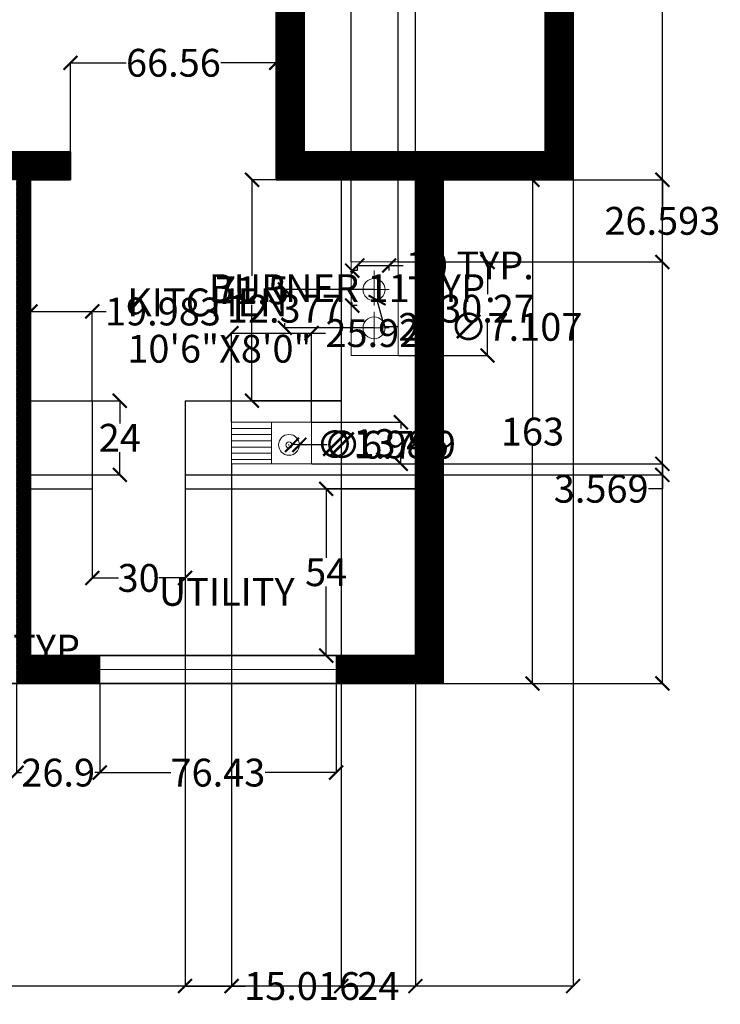
# Model space of a CAD drawing. Units: inches. Extents: x -124 to 468, y -83 to 563.
# Tile 2 of 3: x 241 to 468, y -83 to 235. Entities that reach past the tile are written whole.
import ezdxf

# ---------------------------------------------------------------- set-up
doc = ezdxf.new("R2010")
doc.units = ezdxf.units.IN
doc.header["$MEASUREMENT"] = 0
for name, color, linetype, lineweight in [('A-ANNO-DIMS', 2, 'Continuous', 18), ('A-AREA-IDEN', 7, 'Continuous', 18), ('A-EQPM', 8, 'Continuous', 18), ('A-FLOR-FIXT', 8, 'Continuous', 18)]:
    doc.layers.add(name, color=color, linetype=linetype, lineweight=lineweight)
for name, color, linetype, lineweight, true_color in [('A-FLOR-CASE', 35, 'Continuous', 25, 0x836e59), ('A-GLAZ', 145, 'Continuous', 18, 0x2a88b7), ('A-WALL', 149, 'Continuous', 35, 0x414448), ('A-WALL-PATT', 251, 'Continuous', 13, 0x585a5e)]:
    doc.layers.add(name, color=color, linetype=linetype, lineweight=lineweight, true_color=true_color)
doc.styles.get("Standard").update_dxf_attribs({"font": 'arial.ttf'})
doc.dimstyles.get("Standard").update_dxf_attribs({"dimtxt": 9, "dimasz": 4.5, "dimexe": 0.18, "dimexo": 0.0625, "dimgap": 0.09, "dimtad": 0, "dimtih": 1, "dimtoh": 1, "dimdec": 1, "dimzin": 0, "dimdsep": 46, "dimlunit": 4, "dimtxsty": 'Standard', "dimblk": 'ARCHTICK', "dimcen": 0.09, "dimadec": 0, "dimazin": 0, "dimtfac": 1, "dimtdec": 1, "dimtofl": 0, "dimtmove": 0, "dimatfit": 3, "dimfxl": 1, "dimtolj": 1, "dimtzin": 0, "dimarcsym": 0})

# ---------------------------------------------------------------- blocks, each defined once
blk = doc.blocks.new('COOKTOP-BURNER')
for p, q in [((5.38, 5.19), (5.38, 11.31)), ((5.38, 11.31), (5.38, 5.19)), ((5.38, 5.19), (0, 5.19)), ((5.38, 5.19), (10.26, 5.19)), ((10.26, 5.19), (5.38, 5.19)), ((5.38, 5.19), (5.38, 0)), ((5.38, 0), (5.38, 5.19))]:
    blk.add_line(p, q)
blk.add_circle((5.38, 5.19), 3.55)
blk = doc.blocks.new('_ArchTick')
at = {"color": 0, "linetype": 'ByBlock', "const_width": 0.15}
blk.add_lwpolyline([(-0.5, -0.5), (0.5, 0.5)], dxfattribs=at)
blk = doc.blocks.new('*D6')
at = {"layer": 'A-ANNO-DIMS', "color": 0, "lineweight": -2, "transparency": 16777216}
for p, q in [((39.84, 46.01), (39.84, 31.49)), ((135.84, 46.01), (135.84, 31.49)), ((39.84, 31.67), (135.84, 31.67)), ((135.84, 31.67), (140.34, 31.67))]:
    blk.add_line(p, q, dxfattribs=at)
at = {"layer": 'Defpoints', "color": 0, "transparency": 16777216}
for p in [(39.84, 46.07), (135.84, 46.07), (135.84, 31.67)]:
    blk.add_point(p, dxfattribs=at)
at = {"layer": 'A-ANNO-DIMS', "color": 0, "lineweight": -2, "transparency": 16777216, "xscale": 4.5, "yscale": 4.5, "zscale": 4.5, "rotation": 180}
blk.add_blockref('_ArchTick', (39.84, 31.67), dxfattribs=at)
at = {"layer": 'A-ANNO-DIMS', "color": 0, "lineweight": -2, "transparency": 16777216, "xscale": 4.5, "yscale": 4.5, "zscale": 4.5}
blk.add_blockref('_ArchTick', (135.84, 31.67), dxfattribs=at)
at = {"layer": 'A-ANNO-DIMS', "color": 0, "transparency": 16777216, "insert": (204.38, 31.67), "char_height": 9, "attachment_point": 5}
blk.add_mtext('\\A1;DOUBLE BED 96 TYP.', dxfattribs=at)
blk = doc.blocks.new('*D12')
at = {"layer": 'A-ANNO-DIMS', "color": 0, "lineweight": -2, "transparency": 16777216}
for p, q in [((350.16, 153.98), (348.34, 153.98)), ((348.52, 153.98), (348.52, 153.01)), ((348.52, 142.67), (348.52, 143.64)), ((350.16, 142.67), (348.34, 142.67))]:
    blk.add_line(p, q, dxfattribs=at)
at = {"layer": 'Defpoints', "color": 0, "transparency": 16777216}
for p in [(348.52, 153.98), (350.22, 153.98), (350.22, 142.67)]:
    blk.add_point(p, dxfattribs=at)
at = {"layer": 'A-ANNO-DIMS', "color": 0, "lineweight": -2, "transparency": 16777216, "xscale": 4.5, "yscale": 4.5, "zscale": 4.5}
for p, rotation in [((348.52, 153.98), 90), ((348.52, 142.67), 270)]:
    blk.add_blockref('_ArchTick', p, dxfattribs=dict(at, rotation=rotation))
at = {"layer": 'A-ANNO-DIMS', "color": 0, "transparency": 16777216, "insert": (348.52, 148.32), "char_height": 9, "attachment_point": 5}
blk.add_mtext('\\A1;BURNER 11 TYP.', dxfattribs=at)
blk = doc.blocks.new('*D13')
at = {"layer": 'A-ANNO-DIMS', "color": 0, "lineweight": -2, "transparency": 16777216}
for p, q in [((350.22, 154.04), (350.22, 155.86)), ((350.22, 155.68), (360.48, 155.68)), ((360.48, 154.04), (360.48, 155.86)), ((360.48, 155.68), (364.98, 155.68))]:
    blk.add_line(p, q, dxfattribs=at)
at = {"layer": 'Defpoints', "color": 0, "transparency": 16777216}
for p in [(350.22, 153.98), (360.48, 155.68), (360.48, 153.98)]:
    blk.add_point(p, dxfattribs=at)
at = {"layer": 'A-ANNO-DIMS', "color": 0, "lineweight": -2, "transparency": 16777216, "xscale": 4.5, "yscale": 4.5, "zscale": 4.5, "rotation": 180}
blk.add_blockref('_ArchTick', (350.22, 155.68), dxfattribs=at)
at = {"layer": 'A-ANNO-DIMS', "color": 0, "lineweight": -2, "transparency": 16777216, "xscale": 4.5, "yscale": 4.5, "zscale": 4.5}
blk.add_blockref('_ArchTick', (360.48, 155.68), dxfattribs=at)
at = {"layer": 'A-ANNO-DIMS', "color": 0, "transparency": 16777216, "insert": (386.55, 155.68), "char_height": 9, "attachment_point": 5}
blk.add_mtext('\\A1;10 TYP.', dxfattribs=at)
blk = doc.blocks.new('*D14')
at = {"layer": 'A-ANNO-DIMS', "color": 0, "lineweight": -2, "transparency": 16777216}
for p, q in [((419.98, 183.33), (419.98, -77.73)), ((-79.52, -48.75), (-79.52, -77.73)), ((-79.52, -77.55), (154.74, -77.55)), ((419.98, -77.55), (185.72, -77.55))]:
    blk.add_line(p, q, dxfattribs=at)
at = {"layer": 'Defpoints', "color": 0, "transparency": 16777216}
for p in [(419.98, 183.39), (-79.52, -48.69), (419.98, -77.55)]:
    blk.add_point(p, dxfattribs=at)
at = {"layer": 'A-ANNO-DIMS', "color": 0, "lineweight": -2, "transparency": 16777216, "xscale": 4.5, "yscale": 4.5, "zscale": 4.5, "rotation": 180}
blk.add_blockref('_ArchTick', (-79.52, -77.55), dxfattribs=at)
at = {"layer": 'A-ANNO-DIMS', "color": 0, "lineweight": -2, "transparency": 16777216, "xscale": 4.5, "yscale": 4.5, "zscale": 4.5}
blk.add_blockref('_ArchTick', (419.98, -77.55), dxfattribs=at)
at = {"layer": 'A-ANNO-DIMS', "color": 0, "transparency": 16777216, "insert": (170.23, -77.55), "char_height": 9, "attachment_point": 5}
blk.add_mtext('\\A1;499.5', dxfattribs=at)
blk = doc.blocks.new('*D17')
at = {"layer": 'A-ANNO-DIMS', "color": 0, "lineweight": -2, "transparency": 16777216}
for p, q in [((378.04, 486.39), (449.02, 486.39)), ((448.84, 486.39), (448.84, 258.08)), ((448.84, 20.39), (448.84, 248.71)), ((378.04, 20.39), (449.02, 20.39))]:
    blk.add_line(p, q, dxfattribs=at)
at = {"layer": 'Defpoints', "color": 0, "transparency": 16777216}
for p in [(377.98, 486.39), (448.84, 486.39), (377.98, 20.39)]:
    blk.add_point(p, dxfattribs=at)
at = {"layer": 'A-ANNO-DIMS', "color": 0, "lineweight": -2, "transparency": 16777216, "xscale": 4.5, "yscale": 4.5, "zscale": 4.5}
for p, rotation in [((448.84, 486.39), 90), ((448.84, 20.39), 270)]:
    blk.add_blockref('_ArchTick', p, dxfattribs=dict(at, rotation=rotation))
at = {"layer": 'A-ANNO-DIMS', "color": 0, "transparency": 16777216, "insert": (448.84, 253.39), "char_height": 9, "attachment_point": 5}
blk.add_mtext('\\A1;466', dxfattribs=at)
blk = doc.blocks.new('*D21')
at = {"layer": 'A-ANNO-DIMS', "color": 0, "lineweight": -2, "transparency": 16777216}
for p, q in [((378.04, 183.39), (407.02, 183.39)), ((406.84, 183.39), (406.84, 106.58)), ((406.84, 20.39), (406.84, 97.2)), ((378.04, 20.39), (407.02, 20.39))]:
    blk.add_line(p, q, dxfattribs=at)
at = {"layer": 'Defpoints', "color": 0, "transparency": 16777216}
for p in [(377.98, 183.39), (377.98, 20.39), (406.84, 20.39)]:
    blk.add_point(p, dxfattribs=at)
at = {"layer": 'A-ANNO-DIMS', "color": 0, "lineweight": -2, "transparency": 16777216, "xscale": 4.5, "yscale": 4.5, "zscale": 4.5}
for p, rotation in [((406.84, 183.39), 90), ((406.84, 20.39), 270)]:
    blk.add_blockref('_ArchTick', p, dxfattribs=dict(at, rotation=rotation))
at = {"layer": 'A-ANNO-DIMS', "color": 0, "transparency": 16777216, "insert": (406.84, 101.89), "char_height": 9, "attachment_point": 5}
blk.add_mtext('\\A1;163', dxfattribs=at)
blk = doc.blocks.new('*D31')
at = {"layer": 'A-ANNO-DIMS', "color": 0, "lineweight": -2, "transparency": 16777216}
for p, q in [((239.98, 20.33), (239.98, -8.65)), ((266.88, 20.33), (266.88, -8.65)), ((239.98, -8.47), (241.56, -8.47)), ((266.88, -8.47), (265.29, -8.47))]:
    blk.add_line(p, q, dxfattribs=at)
at = {"layer": 'Defpoints', "color": 0, "transparency": 16777216}
for p in [(239.98, 20.39), (266.88, 20.39), (239.98, -8.47)]:
    blk.add_point(p, dxfattribs=at)
at = {"layer": 'A-ANNO-DIMS', "color": 0, "lineweight": -2, "transparency": 16777216, "xscale": 4.5, "yscale": 4.5, "zscale": 4.5, "rotation": 180.0000000000002}
blk.add_blockref('_ArchTick', (239.98, -8.47), dxfattribs=at)
at = {"layer": 'A-ANNO-DIMS', "color": 0, "lineweight": -2, "transparency": 16777216, "xscale": 4.5, "yscale": 4.5, "zscale": 4.5}
blk.add_blockref('_ArchTick', (266.88, -8.47), dxfattribs=at)
at = {"layer": 'A-ANNO-DIMS', "color": 0, "transparency": 16777216, "insert": (253.43, -8.47), "char_height": 9, "attachment_point": 5}
blk.add_mtext('\\A1;26.9', dxfattribs=at)
blk = doc.blocks.new('*D32')
at = {"layer": 'A-ANNO-DIMS', "color": 0, "lineweight": -2, "transparency": 16777216}
for p, q in [((266.88, 20.33), (266.88, -8.65)), ((343.31, 20.33), (343.31, -8.65)), ((266.88, -8.47), (289.85, -8.47)), ((343.31, -8.47), (320.33, -8.47))]:
    blk.add_line(p, q, dxfattribs=at)
at = {"layer": 'Defpoints', "color": 0, "transparency": 16777216}
for p in [(266.88, 20.39), (343.31, 20.39), (266.88, -8.47)]:
    blk.add_point(p, dxfattribs=at)
at = {"layer": 'A-ANNO-DIMS', "color": 0, "lineweight": -2, "transparency": 16777216, "xscale": 4.5, "yscale": 4.5, "zscale": 4.5, "rotation": 180}
blk.add_blockref('_ArchTick', (266.88, -8.47), dxfattribs=at)
at = {"layer": 'A-ANNO-DIMS', "color": 0, "lineweight": -2, "transparency": 16777216, "xscale": 4.5, "yscale": 4.5, "zscale": 4.5}
blk.add_blockref('_ArchTick', (343.31, -8.47), dxfattribs=at)
at = {"layer": 'A-ANNO-DIMS', "color": 0, "transparency": 16777216, "insert": (305.09, -8.47), "char_height": 9, "attachment_point": 5}
blk.add_mtext('\\A1;76.43', dxfattribs=at)
blk = doc.blocks.new('*D34')
at = {"layer": 'A-ANNO-DIMS', "color": 0, "lineweight": -2, "transparency": 16777216}
for p, q in [((368.91, 83.39), (339.93, 83.39)), ((340.11, 83.39), (340.11, 61.06)), ((340.11, 29.39), (340.11, 51.73)), ((368.91, 29.39), (339.93, 29.39))]:
    blk.add_line(p, q, dxfattribs=at)
at = {"layer": 'Defpoints', "color": 0, "transparency": 16777216}
for p in [(340.11, 83.39), (368.98, 83.39), (368.98, 29.39)]:
    blk.add_point(p, dxfattribs=at)
at = {"layer": 'A-ANNO-DIMS', "color": 0, "lineweight": -2, "transparency": 16777216, "xscale": 4.5, "yscale": 4.5, "zscale": 4.5}
for p, rotation in [((340.11, 83.39), 90), ((340.11, 29.39), 270)]:
    blk.add_blockref('_ArchTick', p, dxfattribs=dict(at, rotation=rotation))
at = {"layer": 'A-ANNO-DIMS', "color": 0, "transparency": 16777216, "insert": (340.11, 56.39), "char_height": 9, "attachment_point": 5}
blk.add_mtext('\\A1;54', dxfattribs=at)
blk = doc.blocks.new('*D47')
at = {"layer": 'A-ANNO-DIMS', "color": 0, "lineweight": -2, "transparency": 16777216}
for p, q in [((264.46, 83.33), (264.46, 54.35)), ((294.46, 83.33), (294.46, 54.35)), ((264.46, 54.53), (272.94, 54.53)), ((294.46, 54.53), (285.98, 54.53))]:
    blk.add_line(p, q, dxfattribs=at)
at = {"layer": 'Defpoints', "color": 0, "transparency": 16777216}
for p in [(264.46, 83.39), (294.46, 83.39), (264.46, 54.53)]:
    blk.add_point(p, dxfattribs=at)
at = {"layer": 'A-ANNO-DIMS', "color": 0, "lineweight": -2, "transparency": 16777216, "xscale": 4.5, "yscale": 4.5, "zscale": 4.5, "rotation": 180}
blk.add_blockref('_ArchTick', (264.46, 54.53), dxfattribs=at)
at = {"layer": 'A-ANNO-DIMS', "color": 0, "lineweight": -2, "transparency": 16777216, "xscale": 4.5, "yscale": 4.5, "zscale": 4.5}
blk.add_blockref('_ArchTick', (294.46, 54.53), dxfattribs=at)
at = {"layer": 'A-ANNO-DIMS', "color": 0, "transparency": 16777216, "insert": (279.46, 54.53), "char_height": 9, "attachment_point": 5}
blk.add_mtext('\\A1;30', dxfattribs=at)
blk = doc.blocks.new('*D48')
at = {"layer": 'A-ANNO-DIMS', "color": 0, "lineweight": -2, "transparency": 16777216}
for p, q in [((344.98, 111.83), (344.98, -77.73)), ((368.98, 83.33), (368.98, -77.73)), ((344.98, -77.55), (350.38, -77.55)), ((368.98, -77.55), (363.57, -77.55))]:
    blk.add_line(p, q, dxfattribs=at)
at = {"layer": 'Defpoints', "color": 0, "transparency": 16777216}
for p in [(344.98, 111.89), (368.98, 83.39), (368.98, -77.55)]:
    blk.add_point(p, dxfattribs=at)
at = {"layer": 'A-ANNO-DIMS', "color": 0, "lineweight": -2, "transparency": 16777216, "xscale": 4.5, "yscale": 4.5, "zscale": 4.5, "rotation": 180}
blk.add_blockref('_ArchTick', (344.98, -77.55), dxfattribs=at)
at = {"layer": 'A-ANNO-DIMS', "color": 0, "lineweight": -2, "transparency": 16777216, "xscale": 4.5, "yscale": 4.5, "zscale": 4.5}
blk.add_blockref('_ArchTick', (368.98, -77.55), dxfattribs=at)
at = {"layer": 'A-ANNO-DIMS', "color": 0, "transparency": 16777216, "insert": (356.98, -77.55), "char_height": 9, "attachment_point": 5}
blk.add_mtext('\\A1;24', dxfattribs=at)
blk = doc.blocks.new('*D49')
at = {"layer": 'A-ANNO-DIMS', "color": 0, "lineweight": -2, "transparency": 16777216}
for p, q in [((257.42, 192.46), (257.42, 221.44)), ((257.42, 221.26), (275.4, 221.26)), ((323.98, 221.26), (306, 221.26)), ((323.98, 192.46), (323.98, 221.44))]:
    blk.add_line(p, q, dxfattribs=at)
at = {"layer": 'Defpoints', "color": 0, "transparency": 16777216}
for p in [(323.98, 221.26), (257.42, 192.39), (323.98, 192.39)]:
    blk.add_point(p, dxfattribs=at)
at = {"layer": 'A-ANNO-DIMS', "color": 0, "lineweight": -2, "transparency": 16777216, "xscale": 4.5, "yscale": 4.5, "zscale": 4.5, "rotation": 180}
blk.add_blockref('_ArchTick', (257.42, 221.26), dxfattribs=at)
at = {"layer": 'A-ANNO-DIMS', "color": 0, "lineweight": -2, "transparency": 16777216, "xscale": 4.5, "yscale": 4.5, "zscale": 4.5}
blk.add_blockref('_ArchTick', (323.98, 221.26), dxfattribs=at)
at = {"layer": 'A-ANNO-DIMS', "color": 0, "transparency": 16777216, "insert": (290.7, 221.26), "char_height": 9, "attachment_point": 5}
blk.add_mtext('\\A1;66.56', dxfattribs=at)
blk = doc.blocks.new('*D50')
at = {"layer": 'A-ANNO-DIMS', "color": 0, "lineweight": -2, "transparency": 16777216}
for p, q in [((244.48, 111.96), (244.48, 140.94)), ((244.48, 140.76), (264.46, 140.76)), ((264.46, 111.96), (264.46, 140.94)), ((264.46, 140.76), (268.96, 140.76))]:
    blk.add_line(p, q, dxfattribs=at)
at = {"layer": 'Defpoints', "color": 0, "transparency": 16777216}
for p in [(264.46, 140.76), (244.48, 111.89), (264.46, 111.89)]:
    blk.add_point(p, dxfattribs=at)
at = {"layer": 'A-ANNO-DIMS', "color": 0, "lineweight": -2, "transparency": 16777216, "xscale": 4.5, "yscale": 4.5, "zscale": 4.5, "rotation": 180}
blk.add_blockref('_ArchTick', (244.48, 140.76), dxfattribs=at)
at = {"layer": 'A-ANNO-DIMS', "color": 0, "lineweight": -2, "transparency": 16777216, "xscale": 4.5, "yscale": 4.5, "zscale": 4.5}
blk.add_blockref('_ArchTick', (264.46, 140.76), dxfattribs=at)
at = {"layer": 'A-ANNO-DIMS', "color": 0, "transparency": 16777216, "insert": (287.31, 140.76), "char_height": 9, "attachment_point": 5}
blk.add_mtext('\\A1;19.983', dxfattribs=at)
blk = doc.blocks.new('*D51')
at = {"layer": 'A-ANNO-DIMS', "color": 0, "lineweight": -2, "transparency": 16777216}
for p, q in [((244.54, 111.89), (273.52, 111.89)), ((273.34, 111.89), (273.34, 104.5)), ((273.34, 87.89), (273.34, 95.28)), ((244.54, 87.89), (273.52, 87.89))]:
    blk.add_line(p, q, dxfattribs=at)
at = {"layer": 'Defpoints', "color": 0, "transparency": 16777216}
for p in [(244.48, 111.89), (244.48, 87.89), (273.34, 87.89)]:
    blk.add_point(p, dxfattribs=at)
at = {"layer": 'A-ANNO-DIMS', "color": 0, "lineweight": -2, "transparency": 16777216, "xscale": 4.5, "yscale": 4.5, "zscale": 4.5}
for p, rotation in [((273.34, 111.89), 90), ((273.34, 87.89), 270)]:
    blk.add_blockref('_ArchTick', p, dxfattribs=dict(at, rotation=rotation))
at = {"layer": 'A-ANNO-DIMS', "color": 0, "transparency": 16777216, "insert": (273.34, 99.89), "char_height": 9, "attachment_point": 5}
blk.add_mtext('\\A1;24', dxfattribs=at)
blk = doc.blocks.new('*D52')
at = {"layer": 'A-ANNO-DIMS', "color": 0, "lineweight": -2, "transparency": 16777216}
for p, q in [((309.48, 91.4), (309.48, -77.73)), ((294.46, 87.83), (294.46, -77.73)), ((294.46, -77.55), (309.48, -77.55)), ((309.48, -77.55), (313.98, -77.55))]:
    blk.add_line(p, q, dxfattribs=at)
at = {"layer": 'Defpoints', "color": 0, "transparency": 16777216}
for p in [(309.48, 91.46), (294.46, 87.89), (309.48, -77.55)]:
    blk.add_point(p, dxfattribs=at)
at = {"layer": 'A-ANNO-DIMS', "color": 0, "lineweight": -2, "transparency": 16777216, "xscale": 4.5, "yscale": 4.5, "zscale": 4.5, "rotation": 180}
blk.add_blockref('_ArchTick', (294.46, -77.55), dxfattribs=at)
at = {"layer": 'A-ANNO-DIMS', "color": 0, "lineweight": -2, "transparency": 16777216, "xscale": 4.5, "yscale": 4.5, "zscale": 4.5}
blk.add_blockref('_ArchTick', (309.48, -77.55), dxfattribs=at)
at = {"layer": 'A-ANNO-DIMS', "color": 0, "transparency": 16777216, "insert": (332.32, -77.55), "char_height": 9, "attachment_point": 5}
blk.add_mtext('\\A1;15.016', dxfattribs=at)
blk = doc.blocks.new('*D53')
at = {"layer": 'A-ANNO-DIMS', "color": 0, "lineweight": -2, "transparency": 16777216}
for p, q in [((309.48, 104.96), (309.48, 133.95)), ((335.39, 104.96), (335.39, 133.95)), ((309.48, 133.77), (335.39, 133.77)), ((335.39, 133.77), (339.89, 133.77))]:
    blk.add_line(p, q, dxfattribs=at)
at = {"layer": 'Defpoints', "color": 0, "transparency": 16777216}
for p in [(335.39, 133.77), (309.48, 104.9), (335.39, 104.9)]:
    blk.add_point(p, dxfattribs=at)
at = {"layer": 'A-ANNO-DIMS', "color": 0, "lineweight": -2, "transparency": 16777216, "xscale": 4.5, "yscale": 4.5, "zscale": 4.5, "rotation": 180}
blk.add_blockref('_ArchTick', (309.48, 133.77), dxfattribs=at)
at = {"layer": 'A-ANNO-DIMS', "color": 0, "lineweight": -2, "transparency": 16777216, "xscale": 4.5, "yscale": 4.5, "zscale": 4.5}
blk.add_blockref('_ArchTick', (335.39, 133.77), dxfattribs=at)
at = {"layer": 'A-ANNO-DIMS', "color": 0, "transparency": 16777216, "insert": (355.2, 133.77), "char_height": 9, "attachment_point": 5}
blk.add_mtext('\\A1;25.92', dxfattribs=at)
blk = doc.blocks.new('*D54')
at = {"layer": 'A-ANNO-DIMS', "color": 0, "lineweight": -2, "transparency": 16777216}
for p, q in [((335.46, 104.9), (364.44, 104.9)), ((364.26, 104.9), (364.26, 102.87)), ((364.26, 91.46), (364.26, 93.49)), ((335.46, 91.46), (364.44, 91.46))]:
    blk.add_line(p, q, dxfattribs=at)
at = {"layer": 'Defpoints', "color": 0, "transparency": 16777216}
for p in [(335.39, 104.9), (335.39, 91.46), (364.26, 91.46)]:
    blk.add_point(p, dxfattribs=at)
at = {"layer": 'A-ANNO-DIMS', "color": 0, "lineweight": -2, "transparency": 16777216, "xscale": 4.5, "yscale": 4.5, "zscale": 4.5}
for p, rotation in [((364.26, 104.9), 90), ((364.26, 91.46), 270)]:
    blk.add_blockref('_ArchTick', p, dxfattribs=dict(at, rotation=rotation))
at = {"layer": 'A-ANNO-DIMS', "color": 0, "transparency": 16777216, "insert": (364.26, 98.18), "char_height": 9, "attachment_point": 5}
blk.add_mtext('\\A1;13.44', dxfattribs=at)
blk = doc.blocks.new('*D55')
at = {"layer": 'A-ANNO-DIMS', "color": 0, "lineweight": -2, "transparency": 16777216}
for p, q in [((335.46, 91.46), (449.02, 91.46)), ((448.84, 91.46), (448.84, 87.89)), ((369.04, 87.89), (449.02, 87.89)), ((448.84, 87.89), (448.84, 83.39)), ((448.84, 83.39), (444.34, 83.39))]:
    blk.add_line(p, q, dxfattribs=at)
at = {"layer": 'Defpoints', "color": 0, "transparency": 16777216}
for p in [(335.39, 91.46), (368.98, 87.89), (448.84, 87.89)]:
    blk.add_point(p, dxfattribs=at)
at = {"layer": 'A-ANNO-DIMS', "color": 0, "lineweight": -2, "transparency": 16777216, "xscale": 4.5, "yscale": 4.5, "zscale": 4.5}
for p, rotation in [((448.84, 91.46), 90), ((448.84, 87.89), 270)]:
    blk.add_blockref('_ArchTick', p, dxfattribs=dict(at, rotation=rotation))
at = {"layer": 'A-ANNO-DIMS', "color": 0, "transparency": 16777216, "insert": (429.06, 83.39), "char_height": 9, "attachment_point": 5}
blk.add_mtext('\\A1;3.569', dxfattribs=at)
blk = doc.blocks.new('*D56')
at = {"layer": 'A-ANNO-DIMS', "color": 0, "lineweight": -2, "transparency": 16777216}
for p, q in [((348.24, 156.86), (348.24, 556.87)), ((348.24, 556.69), (363.44, 556.69)), ((363.44, 156.86), (363.44, 556.87)), ((363.44, 556.69), (367.94, 556.69))]:
    blk.add_line(p, q, dxfattribs=at)
at = {"layer": 'Defpoints', "color": 0, "transparency": 16777216}
for p in [(363.44, 556.69), (348.24, 156.8), (363.44, 156.8)]:
    blk.add_point(p, dxfattribs=at)
at = {"layer": 'A-ANNO-DIMS', "color": 0, "lineweight": -2, "transparency": 16777216, "xscale": 4.5, "yscale": 4.5, "zscale": 4.5, "rotation": 180}
blk.add_blockref('_ArchTick', (348.24, 556.69), dxfattribs=at)
at = {"layer": 'A-ANNO-DIMS', "color": 0, "lineweight": -2, "transparency": 16777216, "xscale": 4.5, "yscale": 4.5, "zscale": 4.5}
blk.add_blockref('_ArchTick', (363.44, 556.69), dxfattribs=at)
at = {"layer": 'A-ANNO-DIMS', "color": 0, "transparency": 16777216, "insert": (386.29, 556.69), "char_height": 9, "attachment_point": 5}
blk.add_mtext('\\A1;15.203', dxfattribs=at)
blk = doc.blocks.new('*D57')
at = {"layer": 'A-ANNO-DIMS', "color": 0, "lineweight": -2, "transparency": 16777216}
for p, q in [((363.5, 156.8), (392.49, 156.8)), ((392.31, 156.8), (392.31, 146.35)), ((392.31, 126.53), (392.31, 136.98)), ((363.5, 126.53), (392.49, 126.53))]:
    blk.add_line(p, q, dxfattribs=at)
at = {"layer": 'Defpoints', "color": 0, "transparency": 16777216}
for p in [(363.44, 156.8), (363.44, 126.53), (392.31, 126.53)]:
    blk.add_point(p, dxfattribs=at)
at = {"layer": 'A-ANNO-DIMS', "color": 0, "lineweight": -2, "transparency": 16777216, "xscale": 4.5, "yscale": 4.5, "zscale": 4.5}
for p, rotation in [((392.31, 156.8), 90), ((392.31, 126.53), 270)]:
    blk.add_blockref('_ArchTick', p, dxfattribs=dict(at, rotation=rotation))
at = {"layer": 'A-ANNO-DIMS', "color": 0, "transparency": 16777216, "insert": (392.31, 141.67), "char_height": 9, "attachment_point": 5}
blk.add_mtext('\\A1;30.27', dxfattribs=at)
blk = doc.blocks.new('*D58')
at = {"layer": 'A-ANNO-DIMS', "color": 0, "lineweight": -2, "transparency": 16777216}
for p, q in [((369.04, 183.39), (449.02, 183.39)), ((448.84, 183.39), (448.84, 174.78)), ((448.84, 156.8), (448.84, 165.41)), ((363.5, 156.8), (449.02, 156.8))]:
    blk.add_line(p, q, dxfattribs=at)
at = {"layer": 'Defpoints', "color": 0, "transparency": 16777216}
for p in [(368.98, 183.39), (363.44, 156.8), (448.84, 156.8)]:
    blk.add_point(p, dxfattribs=at)
at = {"layer": 'A-ANNO-DIMS', "color": 0, "lineweight": -2, "transparency": 16777216, "xscale": 4.5, "yscale": 4.5, "zscale": 4.5}
for p, rotation in [((448.84, 183.39), 90), ((448.84, 156.8), 270)]:
    blk.add_blockref('_ArchTick', p, dxfattribs=dict(at, rotation=rotation))
at = {"layer": 'A-ANNO-DIMS', "color": 0, "transparency": 16777216, "insert": (448.84, 170.1), "char_height": 9, "attachment_point": 5}
blk.add_mtext('\\A1;26.593', dxfattribs=at)
blk = doc.blocks.new('*D59')
at = {"layer": 'A-ANNO-DIMS', "color": 0, "lineweight": -2, "transparency": 16777216}
for p, q in [((363.44, 156.86), (363.44, 556.87)), ((363.44, 556.69), (368.98, 556.69)), ((368.98, 183.46), (368.98, 556.87)), ((368.98, 556.69), (373.48, 556.69))]:
    blk.add_line(p, q, dxfattribs=at)
at = {"layer": 'Defpoints', "color": 0, "transparency": 16777216}
for p in [(368.98, 556.69), (368.98, 183.39), (363.44, 156.8)]:
    blk.add_point(p, dxfattribs=at)
at = {"layer": 'A-ANNO-DIMS', "color": 0, "lineweight": -2, "transparency": 16777216, "xscale": 4.5, "yscale": 4.5, "zscale": 4.5, "rotation": 180}
blk.add_blockref('_ArchTick', (363.44, 556.69), dxfattribs=at)
at = {"layer": 'A-ANNO-DIMS', "color": 0, "lineweight": -2, "transparency": 16777216, "xscale": 4.5, "yscale": 4.5, "zscale": 4.5}
blk.add_blockref('_ArchTick', (368.98, 556.69), dxfattribs=at)
at = {"layer": 'A-ANNO-DIMS', "color": 0, "transparency": 16777216, "insert": (388.79, 556.69), "char_height": 9, "attachment_point": 5}
blk.add_mtext('\\A1;5.535', dxfattribs=at)
blk = doc.blocks.new('*D60')
at = {"layer": 'A-ANNO-DIMS', "color": 0, "lineweight": -2, "transparency": 16777216}
for p, q in [((355.53, 147.85), (326.55, 147.85)), ((326.73, 147.85), (326.73, 146.35)), ((355.53, 135.48), (326.55, 135.48)), ((326.73, 135.48), (326.73, 136.98))]:
    blk.add_line(p, q, dxfattribs=at)
at = {"layer": 'Defpoints', "color": 0, "transparency": 16777216}
for p in [(326.73, 147.85), (355.6, 147.85), (355.6, 135.48)]:
    blk.add_point(p, dxfattribs=at)
at = {"layer": 'A-ANNO-DIMS', "color": 0, "lineweight": -2, "transparency": 16777216, "xscale": 4.5, "yscale": 4.5, "zscale": 4.5}
for p, rotation in [((326.73, 147.85), 90), ((326.73, 135.48), 270)]:
    blk.add_blockref('_ArchTick', p, dxfattribs=dict(at, rotation=rotation))
at = {"layer": 'A-ANNO-DIMS', "color": 0, "transparency": 16777216, "insert": (326.73, 141.67), "char_height": 9, "attachment_point": 5}
blk.add_mtext('\\A1;12.377', dxfattribs=at)
blk = doc.blocks.new('*D61')
at = {"layer": 'A-ANNO-DIMS', "color": 0, "lineweight": -2, "transparency": 16777216}
for p, q in [((344.91, 183.39), (315.93, 183.39)), ((316.11, 183.39), (316.11, 152.33)), ((316.11, 111.89), (316.11, 142.96)), ((344.91, 111.89), (315.93, 111.89))]:
    blk.add_line(p, q, dxfattribs=at)
at = {"layer": 'Defpoints', "color": 0, "transparency": 16777216}
for p in [(316.11, 183.39), (344.98, 183.39), (344.98, 111.89)]:
    blk.add_point(p, dxfattribs=at)
at = {"layer": 'A-ANNO-DIMS', "color": 0, "lineweight": -2, "transparency": 16777216, "xscale": 4.5, "yscale": 4.5, "zscale": 4.5}
for p, rotation in [((316.11, 183.39), 90), ((316.11, 111.89), 270)]:
    blk.add_blockref('_ArchTick', p, dxfattribs=dict(at, rotation=rotation))
at = {"layer": 'A-ANNO-DIMS', "color": 0, "transparency": 16777216, "insert": (316.11, 147.64), "char_height": 9, "attachment_point": 5}
blk.add_mtext('\\A1;71.5', dxfattribs=at)
blk = doc.blocks.new('*D63')
at = {"layer": 'A-ANNO-DIMS', "color": 0, "lineweight": -2, "transparency": 16777216}
for p, q in [((355.51, 147.85), (355.69, 147.85)), ((355.6, 147.76), (355.6, 147.94)), ((359.02, 135.78), (356.56, 144.44)), ((363.52, 135.78), (359.02, 135.78))]:
    blk.add_line(p, q, dxfattribs=at)
at = {"layer": 'Defpoints', "color": 0, "transparency": 16777216}
for p in [(354.63, 151.27), (356.56, 144.44)]:
    blk.add_point(p, dxfattribs=at)
at = {"layer": 'A-ANNO-DIMS', "color": 0, "lineweight": -2, "transparency": 16777216, "xscale": 4.5, "yscale": 4.5, "zscale": 4.5, "rotation": 105.8393017985798}
blk.add_blockref('_ArchTick', (356.56, 144.44), dxfattribs=at)
at = {"layer": 'A-ANNO-DIMS', "color": 0, "transparency": 16777216, "insert": (393.2, 135.78), "char_height": 9, "attachment_point": 5}
blk.add_mtext('\\A1;2X ∅7.107', dxfattribs=at)
blk = doc.blocks.new('*D64')
at = {"layer": 'A-ANNO-DIMS', "color": 0, "lineweight": -2, "transparency": 16777216}
for p, q in [((327.98, 97.59), (328.16, 97.59)), ((328.07, 97.5), (328.07, 97.68)), ((340.43, 97.63), (331.43, 97.6))]:
    blk.add_line(p, q, dxfattribs=at)
at = {"layer": 'Defpoints', "color": 0, "transparency": 16777216}
for p in [(324.72, 97.58), (331.43, 97.6)]:
    blk.add_point(p, dxfattribs=at)
at = {"layer": 'A-ANNO-DIMS', "color": 0, "lineweight": -2, "transparency": 16777216, "xscale": 4.5, "yscale": 4.5, "zscale": 4.5, "rotation": 180.1778218510313}
blk.add_blockref('_ArchTick', (331.43, 97.6), dxfattribs=at)
at = {"layer": 'A-ANNO-DIMS', "color": 0, "transparency": 16777216, "insert": (360.61, 97.63), "char_height": 9, "attachment_point": 5}
blk.add_mtext('\\A1;∅6.719', dxfattribs=at)
blk = doc.blocks.new('*D65')
at = {"layer": 'A-ANNO-DIMS', "color": 0, "lineweight": -2, "transparency": 16777216}
for p, q in [((327.98, 97.59), (328.16, 97.59)), ((328.07, 97.5), (328.07, 97.68)), ((338.07, 97.7), (329.07, 97.6))]:
    blk.add_line(p, q, dxfattribs=at)
at = {"layer": 'Defpoints', "color": 0, "transparency": 16777216}
for p in [(327.08, 97.58), (329.07, 97.6)]:
    blk.add_point(p, dxfattribs=at)
at = {"layer": 'A-ANNO-DIMS', "color": 0, "lineweight": -2, "transparency": 16777216, "xscale": 4.5, "yscale": 4.5, "zscale": 4.5, "rotation": 180.6388736363361}
blk.add_blockref('_ArchTick', (329.07, 97.6), dxfattribs=at)
at = {"layer": 'A-ANNO-DIMS', "color": 0, "transparency": 16777216, "insert": (358.27, 97.7), "char_height": 9, "attachment_point": 5}
blk.add_mtext('\\A1;∅1.985', dxfattribs=at)

msp = doc.modelspace()

# ---------------------------------------------------------------- hatches: boundary and pattern name
at = {"layer": 'A-WALL-PATT'}
h = msp.add_hatch(dxfattribs=at)
h.set_pattern_fill('ANSI31', color=256)
h.set_pattern_definition([(45, (-392.07623, 0), (-0.088388348, 0.088388348), [])])
h.paths.add_polyline_path([(377.9763, 141.7862), (377.9763, 183.3929), (419.9763, 183.3929), (419.9763, 192.3929), (419.9763, 324.3929), (419.9763, 333.3929), (377.9763, 333.3929), (377.9763, 361.0673), (368.9763, 361.0673), (368.9763, 333.3929), (290.9763, 333.3929), (290.9763, 324.3929), (323.9763, 324.3929), (323.9763, 192.3929), (323.9763, 183.3929), (368.9763, 183.3929), (368.9763, 141.7862), (368.9763, 29.3929), (343.3064, 29.3929), (343.3064, 20.3929), (377.9763, 20.3929)])
h.paths.add_polyline_path([(368.9763, 192.3929), (332.9763, 192.3929), (332.9763, 324.3929), (368.9763, 324.3929), (410.9763, 324.3929), (410.9763, 192.3929)], flags=16)
h.paths.add_polyline_path([(215.9763, 29.3929), (179.9763, 29.3929), (179.9763, 75.2245), (175.4763, 75.2245), (175.4763, 29.3929), (167.489, 29.3929), (167.489, 20.3929), (215.9763, 20.3929)])
h.paths.add_polyline_path([(266.8777, 29.3929), (244.4763, 29.3929), (244.4763, 141.7862), (244.4763, 183.3929), (257.421, 183.3929), (257.421, 192.3929), (170.9763, 192.3929), (170.9763, 183.3929), (175.4763, 183.3929), (175.4763, 141.7862), (175.4763, 106.8322), (179.9763, 106.8322), (179.9763, 141.7862), (179.9763, 183.3929), (239.9763, 183.3929), (239.9763, 141.7862), (239.9763, 29.3929), (239.9763, 20.3929), (266.8777, 20.3929)])
h.paths.add_polyline_path([(131.489, 29.3929), (62.8565, 29.3929), (62.8565, 20.3929), (131.489, 20.3929)])
h.paths.add_polyline_path([(26.8565, 29.3929), (-10.5237, 29.3929), (-10.5237, 141.7862), (-10.5237, 183.3929), (125.9763, 183.3929), (125.9763, 192.3929), (-10.5237, 192.3929), (-10.5237, 324.3929), (125.9763, 324.3929), (125.9763, 333.3929), (-10.5237, 333.3929), (-10.5237, 477.3929), (23.4837, 477.3929), (23.4837, 486.3929), (-10.5237, 486.3929), (-10.5237, 527.8228), (-19.5237, 527.8228), (-19.5237, 486.3929), (-19.5237, 264.528), (-79.5237, 264.528), (-79.5237, 255.528), (-19.5237, 255.528), (-19.5237, 156.3747), (-79.5237, 156.3747), (-79.5237, 147.3747), (-19.5237, 147.3747), (-19.5237, 141.7862), (-19.5237, -48.6869), (-10.5237, -48.6869), (-10.5237, 20.3929), (26.8565, 20.3929)])
h.paths.add_polyline_path([(220.4763, 486.3929), (149.9763, 486.3929), (149.9763, 477.3929), (185.9763, 477.3929), (185.9763, 381.3929), (125.9763, 381.3929), (125.9763, 428.759), (121.4763, 428.759), (121.4763, 376.8929), (125.9763, 376.8929), (185.9763, 376.8929), (185.9763, 333.3929), (174.9252, 333.3929), (174.9252, 324.3929), (190.4763, 324.3929), (190.4763, 333.3929), (190.4763, 349.8929), (244.4763, 349.8929), (244.4763, 333.3929), (244.4763, 324.3929), (248.9763, 324.3929), (248.9763, 333.3929), (248.9763, 428.759), (244.4763, 428.759), (244.4763, 354.3929), (190.4763, 354.3929), (190.4763, 477.3929), (220.4763, 477.3929)])
h.paths.add_polyline_path([(377.9763, 486.3929), (310.948, 486.3929), (310.948, 477.3929), (368.9763, 477.3929), (368.9763, 385.0673), (377.9763, 385.0673)])
h.paths.add_polyline_path([(339.1974, 237.2234), (400.8652, 237.2234), (400.8652, 270.8067), (339.1974, 270.8067)], flags=8)
h.paths.add_polyline_path([(182.8614, 357.8948), (247.9303, 357.8948), (247.9303, 391.478), (182.8614, 391.478)], flags=25)

# ---------------------------------------------------------------- linework, layer by layer
at = {"layer": 'A-EQPM'}
for p, q in [((348.2388, 156.7996), (363.4417, 156.7996)), ((348.2388, 126.5317), (348.2388, 156.7996)), ((363.4417, 156.7996), (363.4417, 126.5317)), ((363.4417, 126.5317), (348.2388, 126.5317))]:
    msp.add_line(p, q, dxfattribs=at)
at = {"layer": 'A-FLOR-CASE'}
for p, q in [((344.9763, 183.3929), (344.9763, 141.7862)), ((344.9763, 141.7862), (344.9763, 111.8929)), ((244.4763, 111.8929), (264.4595, 111.8929)), ((264.4595, 111.8929), (264.4595, 83.3929)), ((294.4595, 111.8929), (294.4595, 83.3929)), ((294.4595, 111.8929), (344.9763, 111.8929)), ((244.4763, 87.8929), (264.4595, 87.8929)), ((294.4595, 87.8929), (368.9763, 87.8929)), ((244.4763, 83.3929), (264.4595, 83.3929)), ((294.4595, 83.3929), (368.9763, 83.3929))]:
    msp.add_line(p, q, dxfattribs=at)
at = {"layer": 'A-FLOR-FIXT'}
for p, q in [((309.4756, 104.901), (335.3931, 104.901)), ((309.4756, 91.4618), (309.4756, 104.901)), ((309.4756, 102.901), (322.4343, 102.901)), ((322.4343, 91.4618), (322.4343, 104.901)), ((335.3931, 104.901), (335.3931, 91.4618)), ((309.4756, 100.901), (322.4343, 100.901)), ((309.4756, 98.901), (322.4343, 98.901)), ((309.4756, 96.901), (322.4343, 96.901)), ((309.4756, 94.901), (322.4343, 94.901)), ((309.4756, 92.901), (322.4343, 92.901)), ((335.3931, 91.4618), (309.4756, 91.4618))]:
    msp.add_line(p, q, dxfattribs=at)
for radius in [3.3594, 0.9925]:
    msp.add_circle((328.0744, 97.5897), radius, dxfattribs=at)
at = {"layer": 'A-GLAZ'}
for p, q in [((266.8777, 29.3929), (266.8777, 20.3929)), ((343.3064, 29.3929), (343.3064, 20.3929)), ((266.8777, 24.8929), (343.3064, 24.8929))]:
    msp.add_line(p, q, dxfattribs=at)
at = {"layer": 'A-WALL'}
for p, q in [((323.9763, 324.3929), (323.9763, 192.3929)), ((332.9763, 324.3929), (332.9763, 192.3929)), ((410.9763, 324.3929), (410.9763, 192.3929)), ((419.9763, 324.3929), (419.9763, 192.3929)), ((170.9763, 192.3929), (257.421, 192.3929)), ((257.421, 192.3929), (257.421, 183.3929)), ((323.9763, 192.3929), (323.9763, 183.3929)), ((332.9763, 192.3929), (368.9763, 192.3929)), ((368.9763, 192.3929), (410.9763, 192.3929)), ((419.9763, 192.3929), (419.9763, 183.3929)), ((244.4763, 183.3929), (244.4763, 141.7862)), ((244.4763, 183.3929), (257.421, 183.3929)), ((323.9763, 183.3929), (368.9763, 183.3929)), ((368.9763, 183.3929), (368.9763, 141.7862)), ((377.9763, 183.3929), (419.9763, 183.3929)), ((377.9763, 183.3929), (377.9763, 141.7862)), ((244.4763, 141.7862), (244.4763, 29.3929)), ((368.9763, 141.7862), (368.9763, 29.3929)), ((377.9763, 141.7862), (377.9763, 20.3929)), ((244.4763, 29.3929), (368.9763, 29.3929)), ((-10.5237, 20.3929), (377.9763, 20.3929))]:
    msp.add_line(p, q, dxfattribs=at)

# ---------------------------------------------------------------- block references
at = {"layer": 'A-EQPM'}
msp.add_blockref('COOKTOP-BURNER', (350.218, 142.668), dxfattribs=at)
at = {"layer": 'A-EQPM', "extrusion": (0, 0, -1), "zscale": -1, "rotation": 180}
msp.add_blockref('COOKTOP-BURNER', (-350.218, 140.6633), dxfattribs=at)

# ---------------------------------------------------------------- texts
at = {"layer": 'A-AREA-IDEN', "char_height": 9, "attachment_point": 1}
for s, insert in [('KITCHEN\\P10\'6"X8\'0"', (275.7878, 148.2088)), ('UTILITY', (285.9762, 54.523))]:
    msp.add_mtext_dynamic_manual_height_columns(s, width=177.374172, gutter_width=1, heights=[0], dxfattribs=dict(at, insert=insert))

# ---------------------------------------------------------------- dimensions: what is measured, and where the dimension line sits
at = {"layer": 'A-ANNO-DIMS'}
for base, p1, p2, override, picture, middle in [((363.4417, 556.6878), (348.2388, 156.7996), (363.4417, 156.7996), {"dimdec": 3, "dimlfac": 1, "dimrnd": 0, "dimzin": 0, "dimdsep": 46, "dimlunit": 2}, '*D56', (386.2895, 556.6878)), ((368.9763, 556.6878), (363.4417, 156.7996), (368.9763, 183.3929), {"dimdec": 3, "dimlfac": 1, "dimrnd": 0, "dimzin": 0, "dimdsep": 46, "dimlunit": 2}, '*D59', (388.7853, 556.6878)), ((323.9763, 221.2579), (257.421, 192.3929), (323.9763, 192.3929), {"dimdec": 2, "dimlfac": 1, "dimrnd": 0, "dimzin": 0, "dimdsep": 46, "dimlunit": 2}, '*D49', (290.6986, 221.2579)), ((419.9763, -77.5519), (-79.5237, -48.6869), (419.9763, 183.3929), {"dimdec": 1, "dimlfac": 1, "dimrnd": 0, "dimzin": 0, "dimdsep": 46, "dimlunit": 2}, '*D14', (170.2263, -77.5519)), ((264.4595, 140.7579), (244.4763, 111.8929), (264.4595, 111.8929), {"dimdec": 3, "dimlfac": 1, "dimrnd": 0, "dimzin": 0, "dimdsep": 46, "dimlunit": 2}, '*D50', (287.3073, 140.7579)), ((335.3931, 133.766), (309.4756, 104.901), (335.3931, 104.901), {"dimdec": 2, "dimlfac": 1, "dimrnd": 0, "dimzin": 0, "dimdsep": 46, "dimlunit": 2}, '*D53', (355.199, 133.766)), ((368.9763, -77.5519), (344.9763, 111.8929), (368.9763, 83.3929), {"dimdec": 0, "dimlfac": 1, "dimrnd": 0, "dimzin": 0, "dimdsep": 46, "dimlunit": 2}, '*D48', (356.9763, -77.5519)), ((309.4756, -77.5519), (294.4595, 87.8929), (309.4756, 91.4618), {"dimdec": 3, "dimlfac": 1, "dimrnd": 0, "dimzin": 0, "dimdsep": 46, "dimlunit": 2}, '*D52', (332.3204, -77.5519))]:
    dim = msp.add_linear_dim(base=base, p1=p1, p2=p2, dimstyle='Standard', override=override, dxfattribs=at)
    dim.commit()
    dim.dimension.update_dxf_attribs({"geometry": picture, "text_midpoint": middle})
for base, p1, p2, angle, override, picture, middle in [((448.8413, 486.3929), (377.9763, 20.3929), (377.9763, 486.3929), 90, {"dimdec": 0, "dimlfac": 1, "dimrnd": 0, "dimzin": 0, "dimdsep": 46, "dimlunit": 2}, '*D17', (448.8413, 253.3929)), ((316.1113, 183.3929), (344.9763, 111.8929), (344.9763, 183.3929), 90, {"dimdec": 1, "dimlfac": 1, "dimrnd": 0, "dimzin": 0, "dimdsep": 46, "dimlunit": 2}, '*D61', (316.1113, 147.6429)), ((448.8413, 156.7996), (368.9763, 183.3929), (363.4417, 156.7996), 90, {"dimdec": 3, "dimlfac": 1, "dimrnd": 0, "dimzin": 0, "dimdsep": 46, "dimlunit": 2}, '*D58', (448.8413, 170.0962)), ((406.8413, 20.3929), (377.9763, 183.3929), (377.9763, 20.3929), 270, {"dimdec": 0, "dimlfac": 1, "dimrnd": 0, "dimzin": 0, "dimdsep": 46, "dimlunit": 2}, '*D21', (406.8413, 101.8929)), ((392.3067, 126.5317), (363.4417, 156.7996), (363.4417, 126.5317), 270, {"dimdec": 2, "dimlfac": 1, "dimrnd": 0, "dimzin": 0, "dimdsep": 46, "dimlunit": 2}, '*D57', (392.3067, 141.6656)), ((326.73, 147.854), (355.595, 135.4772), (355.595, 147.854), 90, {"dimdec": 3, "dimlfac": 1, "dimrnd": 0, "dimzin": 0, "dimdsep": 46, "dimlunit": 2}, '*D60', (326.73, 141.6656)), ((273.3413, 87.8929), (244.4763, 111.8929), (244.4763, 87.8929), 270, {"dimdec": 0, "dimlfac": 1, "dimrnd": 0, "dimzin": 0, "dimdsep": 46, "dimlunit": 2}, '*D51', (273.3413, 99.8929)), ((364.2581, 91.4618), (335.3931, 104.901), (335.3931, 91.4618), 270, {"dimdec": 2, "dimlfac": 1, "dimrnd": 0, "dimzin": 0, "dimdsep": 46, "dimlunit": 2}, '*D54', (364.2581, 98.1814)), ((448.8413, 87.8929), (335.3931, 91.4618), (368.9763, 87.8929), 90, {"dimdec": 3, "dimlfac": 1, "dimrnd": 0, "dimzin": 0, "dimdsep": 46, "dimlunit": 2}, '*D55', (429.06, 83.3929)), ((264.4595, 54.5279), (294.4595, 83.3929), (264.4595, 83.3929), 180, {"dimdec": 0, "dimlfac": 1, "dimrnd": 0, "dimzin": 0, "dimdsep": 46, "dimlunit": 2}, '*D47', (279.4595, 54.5279)), ((340.1113, 83.3929), (368.9763, 29.3929), (368.9763, 83.3929), 90, {"dimdec": 0, "dimlfac": 1, "dimrnd": 0, "dimzin": 0, "dimdsep": 46, "dimlunit": 2}, '*D34', (340.1113, 56.3929)), ((239.9763, -8.4721), (266.8777, 20.3929), (239.9763, 20.3929), 180, {"dimdec": 1, "dimlfac": 1, "dimrnd": 0, "dimzin": 0, "dimdsep": 46, "dimlunit": 2}, '*D31', (253.427, -8.4721)), ((266.8777, -8.4721), (343.3064, 20.3929), (266.8777, 20.3929), 180, {"dimdec": 2, "dimlfac": 1, "dimrnd": 0, "dimzin": 0, "dimdsep": 46, "dimlunit": 2}, '*D32', (305.092, -8.4721))]:
    dim = msp.add_linear_dim(base=base, p1=p1, p2=p2, angle=angle, dimstyle='Standard', override=override, dxfattribs=at)
    dim.commit()
    dim.dimension.update_dxf_attribs({"geometry": picture, "text_midpoint": middle})
dim = msp.add_linear_dim(base=(348.5209, 153.9811), p1=(350.2179, 142.6675), p2=(350.2179, 153.9811), angle=90, text='BURNER <> TYP.', dimstyle='Standard', override={"dimdec": 0, "dimlfac": 1, "dimrnd": 0, "dimzin": 0, "dimdsep": 46, "dimlunit": 2}, dxfattribs=at)
dim.commit()
dim.dimension.update_dxf_attribs({"geometry": '*D12', "text_midpoint": (348.5209, 148.3243)})
for base, p1, p2, text, picture, middle in [((360.4787, 155.6782), (350.2179, 153.9811), (360.4787, 153.9811), '<> TYP.', '*D13', (386.5496, 155.6782)), ((135.8352, 31.6703), (39.8352, 46.0703), (135.8352, 46.0703), 'DOUBLE BED <> TYP.', '*D6', (204.3768, 31.6703))]:
    dim = msp.add_linear_dim(base=base, p1=p1, p2=p2, text=text, dimstyle='Standard', override={"dimdec": 0, "dimlfac": 1, "dimrnd": 0, "dimzin": 0, "dimdsep": 46, "dimlunit": 2}, dxfattribs=at)
    dim.commit()
    dim.dimension.update_dxf_attribs({"geometry": picture, "text_midpoint": middle})
dim = msp.add_diameter_dim_2p(p1=(354.6251, 151.2728), p2=(356.565, 144.4352), text='2X <>', dimstyle='Standard', override={"dimdec": 3, "dimlfac": 1, "dimrnd": 0, "dimzin": 0, "dimdsep": 46, "dimlunit": 2}, dxfattribs=at)
dim.commit()
dim.dimension.update_dxf_attribs({"geometry": '*D63', "text_midpoint": (393.1991, 135.7769), "dimtype": 163})
for p1, p2, picture, middle in [((324.715, 97.5793), (331.4337, 97.6001), '*D64', (340.4337, 97.628)), ((327.0819, 97.5786), (329.0669, 97.6007), '*D65', (338.0663, 97.7011))]:
    dim = msp.add_diameter_dim_2p(p1=p1, p2=p2, dimstyle='Standard', override={"dimdec": 3, "dimlfac": 1, "dimrnd": 0, "dimzin": 0, "dimdsep": 46, "dimlunit": 2}, dxfattribs=at)
    dim.commit()
    dim.dimension.update_dxf_attribs({"geometry": picture, "text_midpoint": middle, "dimtype": 163})

doc.saveas('drawing.dxf')
